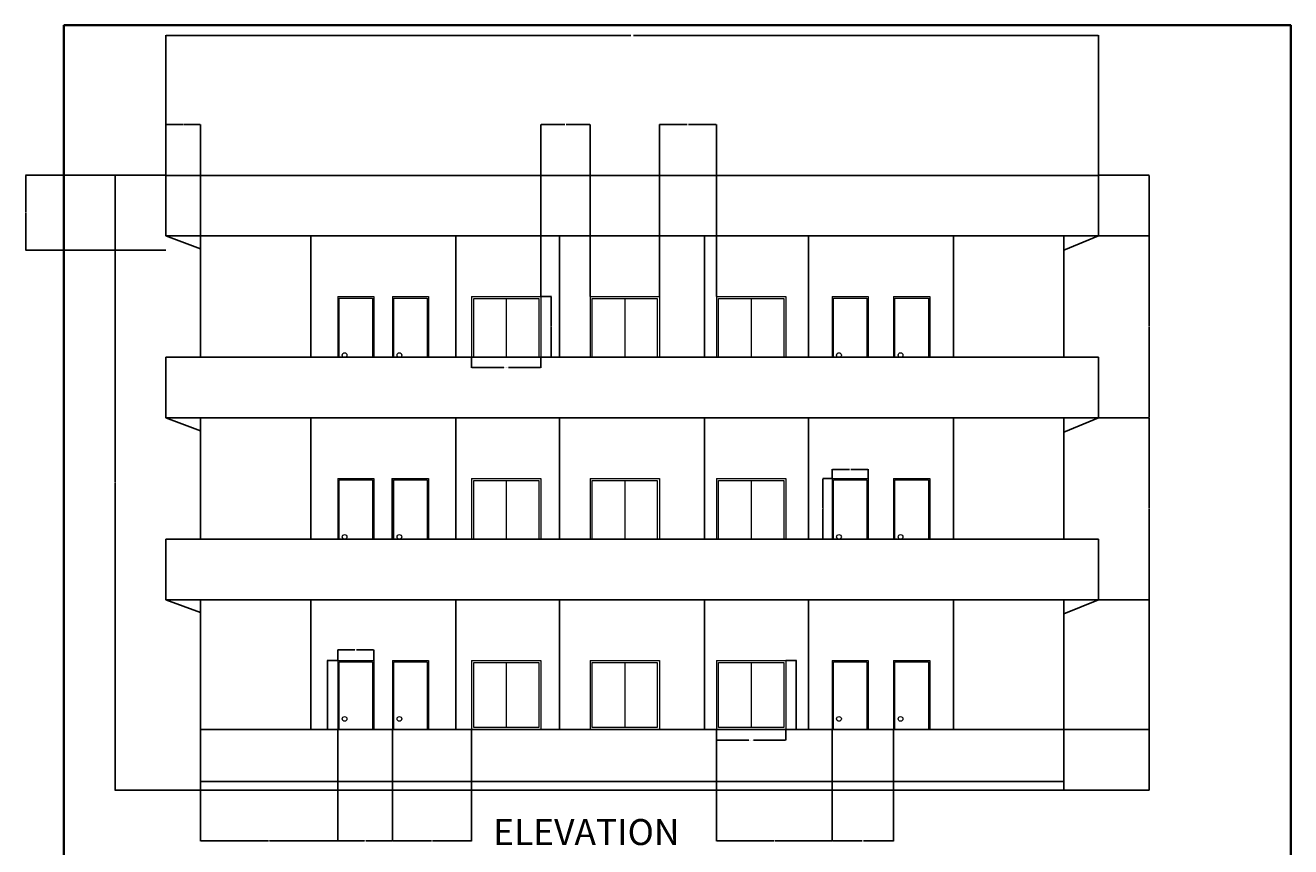
# Model space of a CAD drawing. Units: inches. Extents: x 2165 to 3042, y 1626 to 2968.
# Tile 11 of 11: x 2165 to 3042, y 2399 to 2968. Entities that reach past the tile are written whole.
import ezdxf

# ---------------------------------------------------------------- set-up
doc = ezdxf.new("R2010")
doc.units = ezdxf.units.IN
for name, color, linetype, lineweight in [('A-ANNO-DIMS', 2, 'Continuous', 18), ('A-ANNO-TEXT', 7, 'Continuous', 25), ('A-ELEV', 7, 'Continuous', 25), ('A-ELEV-DOOR', 3, 'Continuous', 18), ('A-ELEV-GLAZ', 4, 'Continuous', 18), ('A-WALL', 7, 'Continuous', 35)]:
    doc.layers.add(name, color=color, linetype=linetype, lineweight=lineweight)
doc.styles.get("Standard").update_dxf_attribs({"font": 'arial.ttf'})
doc.dimstyles.get("Standard").update_dxf_attribs({"dimtxt": 0.18, "dimasz": 0.18, "dimexe": 0.18, "dimexo": 0.0625, "dimgap": 0.09, "dimtad": 0, "dimtih": 1, "dimtoh": 1, "dimdec": 4, "dimzin": 0, "dimdsep": 46, "dimtxsty": 'Standard', "dimcen": 0.09, "dimadec": 0, "dimazin": 0, "dimtfac": 1, "dimtdec": 4, "dimtofl": 0, "dimtmove": 0, "dimatfit": 3, "dimfxl": 1, "dimtolj": 1, "dimtzin": 0, "dimarcsym": 0})

# ---------------------------------------------------------------- blocks, each defined once
blk = doc.blocks.new('ELEV-DOOR-FULL')
for p, q in [((0, 48), (24.97, 48)), ((0, 48), (0, 0)), ((24.97, 48), (24.97, 0))]:
    blk.add_line(p, q)
blk.add_lwpolyline([(0.91, 0), (0.91, 46.97), (24.05, 46.97), (24.05, 0)])
blk.add_circle((4.76, 7.48), 1.64)
blk = doc.blocks.new('ELEV-DOOR-PARTIAL')
for p, q in [((0, 42.16), (24.97, 42.16)), ((0, 42.16), (0, 0.16)), ((24.97, 42.16), (24.97, 0.16))]:
    blk.add_line(p, q)
blk.add_lwpolyline([(0.91, 0.16), (0.91, 41.13), (24.05, 41.13), (24.05, 0.16)])
blk.add_circle((4.76, 1.64), 1.64)
blk = doc.blocks.new('ELEV-WIN-48-SQUARE')
for p, q in [((0, 48), (0, 0)), ((0, 48), (48, 48)), ((24.02, 46.58), (24.02, 1.39)), ((48, 48), (48, 0)), ((0, 0), (48, 0))]:
    blk.add_line(p, q)
blk.add_lwpolyline([(1.46, 46.58), (46.57, 46.58), (46.57, 1.39), (1.46, 1.39)], close=True)
blk = doc.blocks.new('ELEV-WIN-48-PARTIAL')
for p, q in [((0, 42), (0, 0)), ((0, 42), (48, 42)), ((24.02, 40.58), (24.02, 0)), ((48, 42), (48, 0))]:
    blk.add_line(p, q)
blk.add_lwpolyline([(1.46, 0), (1.46, 40.58), (46.57, 40.58), (46.57, 0)])
blk = doc.blocks.new('ELEV-PROJECTING-BAND')
for p, q in [((0, 51.86), (646.5, 51.86)), ((0, 9.86), (0, 51.86)), ((646.5, 9.86), (646.5, 51.86)), ((0, 9.86), (646.5, 9.86)), ((0, 9.86), (24, 0.93)), ((646.5, 9.86), (622.5, 0))]:
    blk.add_line(p, q)
blk = doc.blocks.new('*D40')
at = {"layer": 'A-ANNO-DIMS', "color": 0, "lineweight": -2, "transparency": 16777216}
for p, q in [((2724.42, 2653.94), (2717.98, 2653.94)), ((2718.16, 2653.76), (2718.16, 2633.04)), ((2718.16, 2611.96), (2718.16, 2632.67)), ((2724.42, 2611.78), (2717.98, 2611.78))]:
    blk.add_line(p, q, dxfattribs=at)
at = {"layer": 'A-ANNO-DIMS', "color": 0, "transparency": 16777216}
for points in [[(2718.13, 2653.76), (2718.19, 2653.76), (2718.16, 2653.94)], [(2718.13, 2611.96), (2718.19, 2611.96), (2718.16, 2611.78)]]:
    blk.add_solid(points, dxfattribs=at)
at = {"layer": 'Defpoints', "color": 0, "transparency": 16777216}
for p in [(2718.16, 2653.94), (2724.48, 2653.94), (2724.48, 2611.78)]:
    blk.add_point(p, dxfattribs=at)
at = {"layer": 'A-ANNO-DIMS', "color": 0, "transparency": 16777216, "insert": (2718.16, 2632.86), "char_height": 0.18, "attachment_point": 5}
blk.add_mtext('\\A1;DOOR 42 TYP.', dxfattribs=at)
blk = doc.blocks.new('*D41')
at = {"layer": 'A-ANNO-DIMS', "color": 0, "lineweight": -2, "transparency": 16777216}
for p, q in [((2724.48, 2654), (2724.48, 2660.44)), ((2724.66, 2660.26), (2736.44, 2660.26)), ((2749.27, 2660.26), (2737.5, 2660.26)), ((2749.45, 2654), (2749.45, 2660.44))]:
    blk.add_line(p, q, dxfattribs=at)
at = {"layer": 'A-ANNO-DIMS', "color": 0, "transparency": 16777216}
for points in [[(2724.66, 2660.29), (2724.66, 2660.23), (2724.48, 2660.26)], [(2749.27, 2660.29), (2749.27, 2660.23), (2749.45, 2660.26)]]:
    blk.add_solid(points, dxfattribs=at)
at = {"layer": 'Defpoints', "color": 0, "transparency": 16777216}
for p in [(2749.45, 2660.26), (2724.48, 2653.94), (2749.45, 2653.94)]:
    blk.add_point(p, dxfattribs=at)
at = {"layer": 'A-ANNO-DIMS', "color": 0, "transparency": 16777216, "insert": (2736.97, 2660.26), "char_height": 0.18, "attachment_point": 5}
blk.add_mtext('\\A1;25 TYP.', dxfattribs=at)
blk = doc.blocks.new('*D42')
at = {"layer": 'A-ANNO-DIMS', "color": 0, "lineweight": -2, "transparency": 16777216}
for p, q in [((2474.62, 2737.87), (2474.62, 2730.56)), ((2522.62, 2737.87), (2522.62, 2730.56)), ((2474.8, 2730.74), (2497.04, 2730.74)), ((2522.44, 2730.74), (2500.2, 2730.74))]:
    blk.add_line(p, q, dxfattribs=at)
at = {"layer": 'A-ANNO-DIMS', "color": 0, "transparency": 16777216}
for points in [[(2474.8, 2730.77), (2474.8, 2730.71), (2474.62, 2730.74)], [(2522.44, 2730.77), (2522.44, 2730.71), (2522.62, 2730.74)]]:
    blk.add_solid(points, dxfattribs=at)
at = {"layer": 'Defpoints', "color": 0, "transparency": 16777216}
for p in [(2474.62, 2737.94), (2522.62, 2737.94), (2522.62, 2730.74)]:
    blk.add_point(p, dxfattribs=at)
at = {"layer": 'A-ANNO-DIMS', "color": 0, "transparency": 16777216, "insert": (2498.62, 2730.74), "char_height": 0.18, "attachment_point": 5}
blk.add_mtext('\\A1;UPPER WINDOW 48 TYP.', dxfattribs=at)
blk = doc.blocks.new('*D43')
at = {"layer": 'A-ANNO-DIMS', "color": 0, "lineweight": -2, "transparency": 16777216}
for p, q in [((2522.68, 2779.94), (2530, 2779.94)), ((2529.82, 2779.76), (2529.82, 2759.12)), ((2529.82, 2738.12), (2529.82, 2758.76)), ((2522.68, 2737.94), (2530, 2737.94))]:
    blk.add_line(p, q, dxfattribs=at)
at = {"layer": 'A-ANNO-DIMS', "color": 0, "transparency": 16777216}
for points in [[(2529.79, 2779.76), (2529.85, 2779.76), (2529.82, 2779.94)], [(2529.79, 2738.12), (2529.85, 2738.12), (2529.82, 2737.94)]]:
    blk.add_solid(points, dxfattribs=at)
at = {"layer": 'Defpoints', "color": 0, "transparency": 16777216}
for p in [(2522.62, 2779.94), (2529.82, 2779.94), (2522.62, 2737.94)]:
    blk.add_point(p, dxfattribs=at)
at = {"layer": 'A-ANNO-DIMS', "color": 0, "transparency": 16777216, "insert": (2529.82, 2758.94), "char_height": 0.18, "attachment_point": 5}
blk.add_mtext('\\A1;42 TYP.', dxfattribs=at)
blk = doc.blocks.new('*D44')
at = {"layer": 'A-ANNO-DIMS', "color": 0, "lineweight": -2, "transparency": 16777216}
for p, q in [((2381.72, 2527.94), (2374.41, 2527.94)), ((2374.59, 2527.76), (2374.59, 2504.12)), ((2374.59, 2480.12), (2374.59, 2503.75)), ((2381.72, 2479.94), (2374.41, 2479.94))]:
    blk.add_line(p, q, dxfattribs=at)
at = {"layer": 'A-ANNO-DIMS', "color": 0, "transparency": 16777216}
for points in [[(2374.56, 2527.76), (2374.62, 2527.76), (2374.59, 2527.94)], [(2374.56, 2480.12), (2374.62, 2480.12), (2374.59, 2479.94)]]:
    blk.add_solid(points, dxfattribs=at)
at = {"layer": 'Defpoints', "color": 0, "transparency": 16777216}
for p in [(2374.59, 2527.94), (2381.79, 2527.94), (2381.79, 2479.94)]:
    blk.add_point(p, dxfattribs=at)
at = {"layer": 'A-ANNO-DIMS', "color": 0, "transparency": 16777216, "insert": (2374.59, 2503.94), "char_height": 0.18, "attachment_point": 5}
blk.add_mtext('\\A1;DOOR 48 TYP.', dxfattribs=at)
blk = doc.blocks.new('*D45')
at = {"layer": 'A-ANNO-DIMS', "color": 0, "lineweight": -2, "transparency": 16777216}
for p, q in [((2381.79, 2528), (2381.79, 2535.32)), ((2381.97, 2535.14), (2393.74, 2535.14)), ((2406.57, 2535.14), (2394.8, 2535.14)), ((2406.75, 2528), (2406.75, 2535.32))]:
    blk.add_line(p, q, dxfattribs=at)
at = {"layer": 'A-ANNO-DIMS', "color": 0, "transparency": 16777216}
for points in [[(2381.97, 2535.17), (2381.97, 2535.11), (2381.79, 2535.14)], [(2406.57, 2535.17), (2406.57, 2535.11), (2406.75, 2535.14)]]:
    blk.add_solid(points, dxfattribs=at)
at = {"layer": 'Defpoints', "color": 0, "transparency": 16777216}
for p in [(2406.75, 2535.14), (2381.79, 2527.94), (2406.75, 2527.94)]:
    blk.add_point(p, dxfattribs=at)
at = {"layer": 'A-ANNO-DIMS', "color": 0, "transparency": 16777216, "insert": (2394.27, 2535.14), "char_height": 0.18, "attachment_point": 5}
blk.add_mtext('\\A1;25 TYP.', dxfattribs=at)
blk = doc.blocks.new('*D46')
at = {"layer": 'A-ANNO-DIMS', "color": 0, "lineweight": -2, "transparency": 16777216}
for p, q in [((2644.34, 2479.87), (2644.34, 2472.56)), ((2692.34, 2479.87), (2692.34, 2472.56)), ((2644.52, 2472.74), (2666.73, 2472.74)), ((2692.16, 2472.74), (2669.95, 2472.74))]:
    blk.add_line(p, q, dxfattribs=at)
at = {"layer": 'A-ANNO-DIMS', "color": 0, "transparency": 16777216}
for points in [[(2644.52, 2472.77), (2644.52, 2472.71), (2644.34, 2472.74)], [(2692.16, 2472.77), (2692.16, 2472.71), (2692.34, 2472.74)]]:
    blk.add_solid(points, dxfattribs=at)
at = {"layer": 'Defpoints', "color": 0, "transparency": 16777216}
for p in [(2644.34, 2479.94), (2692.34, 2479.94), (2692.34, 2472.74)]:
    blk.add_point(p, dxfattribs=at)
at = {"layer": 'A-ANNO-DIMS', "color": 0, "transparency": 16777216, "insert": (2668.34, 2472.74), "char_height": 0.18, "attachment_point": 5}
blk.add_mtext('\\A1;LOWER WINDOW 48 TYP.', dxfattribs=at)
blk = doc.blocks.new('*D47')
at = {"layer": 'A-ANNO-DIMS', "color": 0, "lineweight": -2, "transparency": 16777216}
for p, q in [((2692.4, 2527.94), (2699.72, 2527.94)), ((2699.54, 2527.76), (2699.54, 2504.12)), ((2699.54, 2480.12), (2699.54, 2503.75)), ((2692.4, 2479.94), (2699.72, 2479.94))]:
    blk.add_line(p, q, dxfattribs=at)
at = {"layer": 'A-ANNO-DIMS', "color": 0, "transparency": 16777216}
for points in [[(2699.51, 2527.76), (2699.57, 2527.76), (2699.54, 2527.94)], [(2699.51, 2480.12), (2699.57, 2480.12), (2699.54, 2479.94)]]:
    blk.add_solid(points, dxfattribs=at)
at = {"layer": 'Defpoints', "color": 0, "transparency": 16777216}
for p in [(2692.34, 2527.94), (2699.54, 2527.94), (2692.34, 2479.94)]:
    blk.add_point(p, dxfattribs=at)
at = {"layer": 'A-ANNO-DIMS', "color": 0, "transparency": 16777216, "insert": (2699.54, 2503.94), "char_height": 0.18, "attachment_point": 5}
blk.add_mtext('\\A1;48 TYP.', dxfattribs=at)
blk = doc.blocks.new('*D48')
at = {"layer": 'A-ANNO-DIMS', "color": 0, "lineweight": -2, "transparency": 16777216}
for p, q in [((2262.6, 2864), (2262.6, 2961.09)), ((2262.78, 2960.91), (2584.88, 2960.91)), ((2908.92, 2960.91), (2586.83, 2960.91)), ((2909.1, 2864), (2909.1, 2961.09))]:
    blk.add_line(p, q, dxfattribs=at)
at = {"layer": 'A-ANNO-DIMS', "color": 0, "transparency": 16777216}
for points in [[(2262.78, 2960.94), (2262.78, 2960.88), (2262.6, 2960.91)], [(2908.92, 2960.94), (2908.92, 2960.88), (2909.1, 2960.91)]]:
    blk.add_solid(points, dxfattribs=at)
at = {"layer": 'Defpoints', "color": 0, "transparency": 16777216}
for p in [(2909.1, 2960.91), (2262.6, 2863.94), (2909.1, 2863.94)]:
    blk.add_point(p, dxfattribs=at)
at = {"layer": 'A-ANNO-DIMS', "color": 0, "transparency": 16777216, "insert": (2585.85, 2960.91), "char_height": 0.18, "attachment_point": 5}
blk.add_mtext('\\A1;BAND 647 TYP.', dxfattribs=at)
blk = doc.blocks.new('*D49')
at = {"layer": 'A-ANNO-DIMS', "color": 0, "lineweight": -2, "transparency": 16777216}
for p, q in [((2262.54, 2863.94), (2165.45, 2863.94)), ((2165.63, 2863.76), (2165.63, 2838.19)), ((2165.63, 2812.26), (2165.63, 2837.82)), ((2262.54, 2812.08), (2165.45, 2812.08))]:
    blk.add_line(p, q, dxfattribs=at)
at = {"layer": 'A-ANNO-DIMS', "color": 0, "transparency": 16777216}
for points in [[(2165.6, 2863.76), (2165.66, 2863.76), (2165.63, 2863.94)], [(2165.6, 2812.26), (2165.66, 2812.26), (2165.63, 2812.08)]]:
    blk.add_solid(points, dxfattribs=at)
at = {"layer": 'Defpoints', "color": 0, "transparency": 16777216}
for p in [(2165.63, 2863.94), (2262.6, 2863.94), (2262.6, 2812.08)]:
    blk.add_point(p, dxfattribs=at)
at = {"layer": 'A-ANNO-DIMS', "color": 0, "transparency": 16777216, "insert": (2165.63, 2838.01), "char_height": 0.18, "attachment_point": 5}
blk.add_mtext('\\A1;52 TYP.', dxfattribs=at)
blk = doc.blocks.new('*D64')
at = {"layer": 'A-ANNO-DIMS', "color": 0, "lineweight": -2, "transparency": 16777216}
for p, q in [((2262.54, 2863.94), (2227.32, 2863.94)), ((2227.5, 2863.76), (2227.5, 2651.12)), ((2227.5, 2438.12), (2227.5, 2650.75)), ((2286.54, 2437.94), (2227.32, 2437.94))]:
    blk.add_line(p, q, dxfattribs=at)
at = {"layer": 'A-ANNO-DIMS', "color": 0, "transparency": 16777216}
for points in [[(2227.47, 2863.76), (2227.53, 2863.76), (2227.5, 2863.94)], [(2227.47, 2438.12), (2227.53, 2438.12), (2227.5, 2437.94)]]:
    blk.add_solid(points, dxfattribs=at)
at = {"layer": 'Defpoints', "color": 0, "transparency": 16777216}
for p in [(2227.5, 2863.94), (2262.6, 2863.94), (2286.6, 2437.94)]:
    blk.add_point(p, dxfattribs=at)
at = {"layer": 'A-ANNO-DIMS', "color": 0, "transparency": 16777216, "insert": (2227.5, 2650.94), "char_height": 0.18, "attachment_point": 5}
blk.add_mtext('\\A1;426', dxfattribs=at)
blk = doc.blocks.new('*D65')
at = {"layer": 'A-ANNO-DIMS', "color": 0, "lineweight": -2, "transparency": 16777216}
for p, q in [((2885.17, 2479.94), (2944.38, 2479.94)), ((2944.2, 2479.76), (2944.2, 2459.12)), ((2944.2, 2438.12), (2944.2, 2458.76)), ((2885.17, 2437.94), (2944.38, 2437.94))]:
    blk.add_line(p, q, dxfattribs=at)
at = {"layer": 'A-ANNO-DIMS', "color": 0, "transparency": 16777216}
for points in [[(2944.17, 2479.76), (2944.23, 2479.76), (2944.2, 2479.94)], [(2944.17, 2438.12), (2944.23, 2438.12), (2944.2, 2437.94)]]:
    blk.add_solid(points, dxfattribs=at)
at = {"layer": 'Defpoints', "color": 0, "transparency": 16777216}
for p in [(2885.1, 2479.94), (2944.2, 2479.94), (2885.1, 2437.94)]:
    blk.add_point(p, dxfattribs=at)
at = {"layer": 'A-ANNO-DIMS', "color": 0, "transparency": 16777216, "insert": (2944.2, 2458.94), "char_height": 0.18, "attachment_point": 5}
blk.add_mtext('\\A1;42', dxfattribs=at)
blk = doc.blocks.new('*D66')
at = {"layer": 'A-ANNO-DIMS', "color": 0, "lineweight": -2, "transparency": 16777216}
for p, q in [((2909.17, 2569.94), (2944.38, 2569.94)), ((2944.2, 2569.76), (2944.2, 2525.12)), ((2944.2, 2480.12), (2944.2, 2524.75)), ((2885.17, 2479.94), (2944.38, 2479.94))]:
    blk.add_line(p, q, dxfattribs=at)
at = {"layer": 'A-ANNO-DIMS', "color": 0, "transparency": 16777216}
for points in [[(2944.17, 2569.76), (2944.23, 2569.76), (2944.2, 2569.94)], [(2944.17, 2480.12), (2944.23, 2480.12), (2944.2, 2479.94)]]:
    blk.add_solid(points, dxfattribs=at)
at = {"layer": 'Defpoints', "color": 0, "transparency": 16777216}
for p in [(2909.1, 2569.94), (2944.2, 2569.94), (2885.1, 2479.94)]:
    blk.add_point(p, dxfattribs=at)
at = {"layer": 'A-ANNO-DIMS', "color": 0, "transparency": 16777216, "insert": (2944.2, 2524.94), "char_height": 0.18, "attachment_point": 5}
blk.add_mtext('\\A1;90', dxfattribs=at)
blk = doc.blocks.new('*D67')
at = {"layer": 'A-ANNO-DIMS', "color": 0, "lineweight": -2, "transparency": 16777216}
for p, q in [((2909.17, 2695.94), (2944.38, 2695.94)), ((2944.2, 2695.76), (2944.2, 2633.12)), ((2944.2, 2570.12), (2944.2, 2632.75)), ((2909.17, 2569.94), (2944.38, 2569.94))]:
    blk.add_line(p, q, dxfattribs=at)
at = {"layer": 'A-ANNO-DIMS', "color": 0, "transparency": 16777216}
for points in [[(2944.17, 2695.76), (2944.23, 2695.76), (2944.2, 2695.94)], [(2944.17, 2570.12), (2944.23, 2570.12), (2944.2, 2569.94)]]:
    blk.add_solid(points, dxfattribs=at)
at = {"layer": 'Defpoints', "color": 0, "transparency": 16777216}
for p in [(2909.1, 2695.94), (2944.2, 2695.94), (2909.1, 2569.94)]:
    blk.add_point(p, dxfattribs=at)
at = {"layer": 'A-ANNO-DIMS', "color": 0, "transparency": 16777216, "insert": (2944.2, 2632.94), "char_height": 0.18, "attachment_point": 5}
blk.add_mtext('\\A1;126', dxfattribs=at)
blk = doc.blocks.new('*D68')
at = {"layer": 'A-ANNO-DIMS', "color": 0, "lineweight": -2, "transparency": 16777216}
for p, q in [((2909.17, 2821.94), (2944.38, 2821.94)), ((2944.2, 2821.76), (2944.2, 2759.12)), ((2944.2, 2696.12), (2944.2, 2758.75)), ((2909.17, 2695.94), (2944.38, 2695.94))]:
    blk.add_line(p, q, dxfattribs=at)
at = {"layer": 'A-ANNO-DIMS', "color": 0, "transparency": 16777216}
for points in [[(2944.17, 2821.76), (2944.23, 2821.76), (2944.2, 2821.94)], [(2944.17, 2696.12), (2944.23, 2696.12), (2944.2, 2695.94)]]:
    blk.add_solid(points, dxfattribs=at)
at = {"layer": 'Defpoints', "color": 0, "transparency": 16777216}
for p in [(2909.1, 2821.94), (2944.2, 2821.94), (2909.1, 2695.94)]:
    blk.add_point(p, dxfattribs=at)
at = {"layer": 'A-ANNO-DIMS', "color": 0, "transparency": 16777216, "insert": (2944.2, 2758.94), "char_height": 0.18, "attachment_point": 5}
blk.add_mtext('\\A1;126', dxfattribs=at)
blk = doc.blocks.new('*D69')
at = {"layer": 'A-ANNO-DIMS', "color": 0, "lineweight": -2, "transparency": 16777216}
for p, q in [((2909.17, 2863.94), (2944.38, 2863.94)), ((2944.2, 2863.76), (2944.2, 2843.12)), ((2944.2, 2822.12), (2944.2, 2842.76)), ((2909.17, 2821.94), (2944.38, 2821.94))]:
    blk.add_line(p, q, dxfattribs=at)
at = {"layer": 'A-ANNO-DIMS', "color": 0, "transparency": 16777216}
for points in [[(2944.17, 2863.76), (2944.23, 2863.76), (2944.2, 2863.94)], [(2944.17, 2822.12), (2944.23, 2822.12), (2944.2, 2821.94)]]:
    blk.add_solid(points, dxfattribs=at)
at = {"layer": 'Defpoints', "color": 0, "transparency": 16777216}
for p in [(2909.1, 2863.94), (2944.2, 2863.94), (2909.1, 2821.94)]:
    blk.add_point(p, dxfattribs=at)
at = {"layer": 'A-ANNO-DIMS', "color": 0, "transparency": 16777216, "insert": (2944.2, 2842.94), "char_height": 0.18, "attachment_point": 5}
blk.add_mtext('\\A1;42', dxfattribs=at)
blk = doc.blocks.new('*D70')
at = {"layer": 'A-ANNO-DIMS', "color": 0, "lineweight": -2, "transparency": 16777216}
for p, q in [((2262.6, 2822), (2262.6, 2899.22)), ((2262.78, 2899.04), (2274.38, 2899.04)), ((2286.42, 2899.04), (2274.82, 2899.04)), ((2286.6, 2813.07), (2286.6, 2899.22))]:
    blk.add_line(p, q, dxfattribs=at)
at = {"layer": 'A-ANNO-DIMS', "color": 0, "transparency": 16777216}
for points in [[(2262.78, 2899.07), (2262.78, 2899.01), (2262.6, 2899.04)], [(2286.42, 2899.07), (2286.42, 2899.01), (2286.6, 2899.04)]]:
    blk.add_solid(points, dxfattribs=at)
at = {"layer": 'Defpoints', "color": 0, "transparency": 16777216}
for p in [(2286.6, 2899.04), (2262.6, 2821.94), (2286.6, 2813.01)]:
    blk.add_point(p, dxfattribs=at)
at = {"layer": 'A-ANNO-DIMS', "color": 0, "transparency": 16777216, "insert": (2274.6, 2899.04), "char_height": 0.18, "attachment_point": 5}
blk.add_mtext('\\A1;24', dxfattribs=at)
blk = doc.blocks.new('*D71')
at = {"layer": 'A-ANNO-DIMS', "color": 0, "lineweight": -2, "transparency": 16777216}
for p, q in [((2381.79, 2479.87), (2381.79, 2402.66)), ((2286.6, 2437.87), (2286.6, 2402.66)), ((2286.78, 2402.84), (2333.8, 2402.84)), ((2381.61, 2402.84), (2334.59, 2402.84))]:
    blk.add_line(p, q, dxfattribs=at)
at = {"layer": 'A-ANNO-DIMS', "color": 0, "transparency": 16777216}
for points in [[(2286.78, 2402.87), (2286.78, 2402.81), (2286.6, 2402.84)], [(2381.61, 2402.87), (2381.61, 2402.81), (2381.79, 2402.84)]]:
    blk.add_solid(points, dxfattribs=at)
at = {"layer": 'Defpoints', "color": 0, "transparency": 16777216}
for p in [(2381.79, 2479.94), (2286.6, 2437.94), (2381.79, 2402.84)]:
    blk.add_point(p, dxfattribs=at)
at = {"layer": 'A-ANNO-DIMS', "color": 0, "transparency": 16777216, "insert": (2334.19, 2402.84), "char_height": 0.18, "attachment_point": 5}
blk.add_mtext('\\A1;95.18', dxfattribs=at)
blk = doc.blocks.new('*D72')
at = {"layer": 'A-ANNO-DIMS', "color": 0, "lineweight": -2, "transparency": 16777216}
for p, q in [((2381.79, 2479.87), (2381.79, 2402.66)), ((2419.77, 2479.87), (2419.77, 2402.66)), ((2381.97, 2402.84), (2400.38, 2402.84)), ((2419.59, 2402.84), (2401.17, 2402.84))]:
    blk.add_line(p, q, dxfattribs=at)
at = {"layer": 'A-ANNO-DIMS', "color": 0, "transparency": 16777216}
for points in [[(2381.97, 2402.87), (2381.97, 2402.81), (2381.79, 2402.84)], [(2419.59, 2402.87), (2419.59, 2402.81), (2419.77, 2402.84)]]:
    blk.add_solid(points, dxfattribs=at)
at = {"layer": 'Defpoints', "color": 0, "transparency": 16777216}
for p in [(2381.79, 2479.94), (2419.77, 2479.94), (2419.77, 2402.84)]:
    blk.add_point(p, dxfattribs=at)
at = {"layer": 'A-ANNO-DIMS', "color": 0, "transparency": 16777216, "insert": (2400.78, 2402.84), "char_height": 0.18, "attachment_point": 5}
blk.add_mtext('\\A1;37.99', dxfattribs=at)
blk = doc.blocks.new('*D73')
at = {"layer": 'A-ANNO-DIMS', "color": 0, "lineweight": -2, "transparency": 16777216}
for p, q in [((2419.77, 2479.87), (2419.77, 2402.66)), ((2474.62, 2479.87), (2474.62, 2402.66)), ((2419.95, 2402.84), (2446.8, 2402.84)), ((2474.44, 2402.84), (2447.59, 2402.84))]:
    blk.add_line(p, q, dxfattribs=at)
at = {"layer": 'A-ANNO-DIMS', "color": 0, "transparency": 16777216}
for points in [[(2419.95, 2402.87), (2419.95, 2402.81), (2419.77, 2402.84)], [(2474.44, 2402.87), (2474.44, 2402.81), (2474.62, 2402.84)]]:
    blk.add_solid(points, dxfattribs=at)
at = {"layer": 'Defpoints', "color": 0, "transparency": 16777216}
for p in [(2419.77, 2479.94), (2474.62, 2479.94), (2474.62, 2402.84)]:
    blk.add_point(p, dxfattribs=at)
at = {"layer": 'A-ANNO-DIMS', "color": 0, "transparency": 16777216, "insert": (2447.2, 2402.84), "char_height": 0.18, "attachment_point": 5}
blk.add_mtext('\\A1;54.85', dxfattribs=at)
blk = doc.blocks.new('*D74')
at = {"layer": 'A-ANNO-DIMS', "color": 0, "lineweight": -2, "transparency": 16777216}
for p, q in [((2522.62, 2780), (2522.62, 2899.22)), ((2522.8, 2899.04), (2539.21, 2899.04)), ((2556.55, 2899.04), (2540.14, 2899.04)), ((2556.73, 2780), (2556.73, 2899.22))]:
    blk.add_line(p, q, dxfattribs=at)
at = {"layer": 'A-ANNO-DIMS', "color": 0, "transparency": 16777216}
for points in [[(2522.8, 2899.07), (2522.8, 2899.01), (2522.62, 2899.04)], [(2556.55, 2899.07), (2556.55, 2899.01), (2556.73, 2899.04)]]:
    blk.add_solid(points, dxfattribs=at)
at = {"layer": 'Defpoints', "color": 0, "transparency": 16777216}
for p in [(2556.73, 2899.04), (2522.62, 2779.94), (2556.73, 2779.94)]:
    blk.add_point(p, dxfattribs=at)
at = {"layer": 'A-ANNO-DIMS', "color": 0, "transparency": 16777216, "insert": (2539.67, 2899.04), "char_height": 0.18, "attachment_point": 5}
blk.add_mtext('\\A1;34.104', dxfattribs=at)
blk = doc.blocks.new('*D75')
at = {"layer": 'A-ANNO-DIMS', "color": 0, "lineweight": -2, "transparency": 16777216}
for p, q in [((2604.73, 2780), (2604.73, 2899.22)), ((2604.91, 2899.04), (2624.07, 2899.04)), ((2644.16, 2899.04), (2625, 2899.04)), ((2644.34, 2780), (2644.34, 2899.22))]:
    blk.add_line(p, q, dxfattribs=at)
at = {"layer": 'A-ANNO-DIMS', "color": 0, "transparency": 16777216}
for points in [[(2604.91, 2899.07), (2604.91, 2899.01), (2604.73, 2899.04)], [(2644.16, 2899.07), (2644.16, 2899.01), (2644.34, 2899.04)]]:
    blk.add_solid(points, dxfattribs=at)
at = {"layer": 'Defpoints', "color": 0, "transparency": 16777216}
for p in [(2644.34, 2899.04), (2604.73, 2779.94), (2644.34, 2779.94)]:
    blk.add_point(p, dxfattribs=at)
at = {"layer": 'A-ANNO-DIMS', "color": 0, "transparency": 16777216, "insert": (2624.53, 2899.04), "char_height": 0.18, "attachment_point": 5}
blk.add_mtext('\\A1;39.615', dxfattribs=at)
blk = doc.blocks.new('*D76')
at = {"layer": 'A-ANNO-DIMS', "color": 0, "lineweight": -2, "transparency": 16777216}
for p, q in [((2644.34, 2479.87), (2644.34, 2402.66)), ((2724.48, 2479.87), (2724.48, 2402.66)), ((2644.52, 2402.84), (2684.02, 2402.84)), ((2724.3, 2402.84), (2684.81, 2402.84))]:
    blk.add_line(p, q, dxfattribs=at)
at = {"layer": 'A-ANNO-DIMS', "color": 0, "transparency": 16777216}
for points in [[(2644.52, 2402.87), (2644.52, 2402.81), (2644.34, 2402.84)], [(2724.3, 2402.87), (2724.3, 2402.81), (2724.48, 2402.84)]]:
    blk.add_solid(points, dxfattribs=at)
at = {"layer": 'Defpoints', "color": 0, "transparency": 16777216}
for p in [(2644.34, 2479.94), (2724.48, 2479.94), (2724.48, 2402.84)]:
    blk.add_point(p, dxfattribs=at)
at = {"layer": 'A-ANNO-DIMS', "color": 0, "transparency": 16777216, "insert": (2684.41, 2402.84), "char_height": 0.18, "attachment_point": 5}
blk.add_mtext('\\A1;80.14', dxfattribs=at)
blk = doc.blocks.new('*D77')
at = {"layer": 'A-ANNO-DIMS', "color": 0, "lineweight": -2, "transparency": 16777216}
for p, q in [((2724.48, 2479.87), (2724.48, 2402.66)), ((2767.15, 2479.87), (2767.15, 2402.66)), ((2724.66, 2402.84), (2745.42, 2402.84)), ((2766.97, 2402.84), (2746.21, 2402.84))]:
    blk.add_line(p, q, dxfattribs=at)
at = {"layer": 'A-ANNO-DIMS', "color": 0, "transparency": 16777216}
for points in [[(2724.66, 2402.87), (2724.66, 2402.81), (2724.48, 2402.84)], [(2766.97, 2402.87), (2766.97, 2402.81), (2767.15, 2402.84)]]:
    blk.add_solid(points, dxfattribs=at)
at = {"layer": 'Defpoints', "color": 0, "transparency": 16777216}
for p in [(2724.48, 2479.94), (2767.15, 2479.94), (2767.15, 2402.84)]:
    blk.add_point(p, dxfattribs=at)
at = {"layer": 'A-ANNO-DIMS', "color": 0, "transparency": 16777216, "insert": (2745.82, 2402.84), "char_height": 0.18, "attachment_point": 5}
blk.add_mtext('\\A1;42.66', dxfattribs=at)

msp = doc.modelspace()

# ---------------------------------------------------------------- linework, layer by layer
at = {"layer": 'A-ELEV'}
for p, q in [((2286.6045, 2821.9361), (2286.6045, 2737.9361)), ((2363.1045, 2821.9361), (2363.1045, 2737.9361)), ((2463.6045, 2821.9361), (2463.6045, 2737.9361)), ((2535.6045, 2821.9361), (2535.6045, 2737.9361)), ((2636.1045, 2821.9361), (2636.1045, 2737.9361)), ((2708.1045, 2821.9361), (2708.1045, 2737.9361)), ((2708.1045, 2821.9361), (2708.1045, 2737.9361)), ((2808.6045, 2821.9361), (2808.6045, 2737.9361)), ((2808.6045, 2821.9361), (2808.6045, 2737.9361)), ((2885.1045, 2821.9361), (2885.1045, 2737.9361)), ((2286.6045, 2695.9361), (2286.6045, 2611.9361)), ((2286.6045, 2695.9361), (2286.6045, 2689.9361)), ((2363.1045, 2695.9361), (2363.1045, 2611.9361)), ((2463.6045, 2695.9361), (2463.6045, 2611.9361)), ((2535.6045, 2695.9361), (2535.6045, 2611.9361)), ((2636.1045, 2695.9361), (2636.1045, 2611.9361)), ((2708.1045, 2695.9361), (2708.1045, 2611.9361)), ((2708.1045, 2695.9361), (2708.1045, 2611.9361)), ((2808.6045, 2695.9361), (2808.6045, 2611.9361)), ((2808.6045, 2695.9361), (2808.6045, 2611.9361)), ((2885.1045, 2695.9361), (2885.1045, 2611.9361)), ((2885.1045, 2695.9361), (2885.1045, 2689.9361)), ((2286.6045, 2569.9361), (2286.6045, 2437.9361)), ((2286.6045, 2569.9361), (2286.6045, 2563.9361)), ((2363.1045, 2569.9361), (2363.1045, 2479.9361)), ((2463.6045, 2569.9361), (2463.6045, 2479.9361)), ((2535.6045, 2569.9361), (2535.6045, 2479.9361)), ((2636.1045, 2569.9361), (2636.1045, 2479.9361)), ((2708.1045, 2569.9361), (2708.1045, 2479.9361)), ((2708.1045, 2569.9361), (2708.1045, 2479.9361)), ((2808.6045, 2569.9361), (2808.6045, 2479.9361)), ((2808.6045, 2569.9361), (2808.6045, 2479.9361)), ((2885.1045, 2569.9361), (2885.1045, 2437.9361)), ((2885.1045, 2569.9361), (2885.1045, 2563.9361)), ((2363.1045, 2479.9361), (2286.6045, 2479.9361)), ((2286.6045, 2479.9361), (2885.1045, 2479.9361)), ((2363.1045, 2479.9361), (2463.6045, 2479.9361)), ((2708.1045, 2479.9361), (2808.6045, 2479.9361)), ((2286.6045, 2443.9361), (2885.1045, 2443.9361)), ((2286.6045, 2437.9361), (2885.1045, 2437.9361))]:
    msp.add_line(p, q, dxfattribs=at)
at = {"layer": 'A-ELEV-DOOR'}
for p, q in [((2381.7854, 2779.9361), (2406.7549, 2779.9361)), ((2406.7549, 2779.9361), (2406.7549, 2737.9361)), ((2419.7722, 2779.9361), (2444.7417, 2779.9361)), ((2444.7417, 2779.9361), (2444.7417, 2737.9361)), ((2767.1472, 2779.9361), (2792.1167, 2779.9361)), ((2792.1167, 2779.9361), (2792.1167, 2737.9361)), ((2381.7854, 2653.9361), (2406.7549, 2653.9361)), ((2406.7549, 2653.9361), (2406.7549, 2611.9361)), ((2419.2885, 2653.9361), (2419.2885, 2611.9361)), ((2419.2885, 2653.9361), (2444.7417, 2653.9361)), ((2444.7417, 2653.9361), (2444.7417, 2611.9361)), ((2767.1472, 2653.9361), (2792.1167, 2653.9361)), ((2792.1167, 2653.9361), (2792.1167, 2611.9361)), ((2381.7854, 2527.9361), (2406.7549, 2527.9361)), ((2406.7549, 2527.9361), (2406.7549, 2479.9361)), ((2419.7722, 2527.9361), (2444.7417, 2527.9361)), ((2444.7417, 2527.9361), (2444.7417, 2479.9361)), ((2767.1472, 2527.9361), (2792.1167, 2527.9361)), ((2792.1167, 2527.9361), (2792.1167, 2479.9361))]:
    msp.add_line(p, q, dxfattribs=at)
at = {"layer": 'A-ELEV-GLAZ'}
for p, q in [((2556.726, 2779.9361), (2556.726, 2737.9361)), ((2556.726, 2779.9361), (2604.726, 2779.9361)), ((2604.726, 2779.9361), (2604.726, 2737.9361)), ((2644.3411, 2779.9361), (2644.3411, 2737.9361)), ((2644.3411, 2779.9361), (2692.3411, 2779.9361)), ((2692.3411, 2779.9361), (2692.3411, 2737.9361)), ((2556.726, 2653.9361), (2556.726, 2611.9361)), ((2556.726, 2653.9361), (2604.726, 2653.9361)), ((2604.726, 2653.9361), (2604.726, 2611.9361)), ((2644.3411, 2653.9361), (2644.3411, 2611.9361)), ((2644.3411, 2653.9361), (2692.3411, 2653.9361)), ((2692.3411, 2653.9361), (2692.3411, 2611.9361)), ((2556.726, 2527.9361), (2556.726, 2479.9361)), ((2556.726, 2527.9361), (2604.726, 2527.9361)), ((2604.726, 2527.9361), (2604.726, 2479.9361)), ((2644.3411, 2527.9361), (2644.3411, 2479.9361)), ((2644.3411, 2527.9361), (2692.3411, 2527.9361)), ((2692.3411, 2527.9361), (2692.3411, 2479.9361)), ((2556.726, 2479.9361), (2604.726, 2479.9361)), ((2644.3411, 2479.9361), (2692.3411, 2479.9361))]:
    msp.add_line(p, q, dxfattribs=at)
at = {"layer": 'A-WALL'}
msp.add_lwpolyline([(2191.9961, 2967.8547), (3042.3708, 2967.8547), (3042.3708, 1626.3264), (2191.9961, 1626.3264)], close=True, dxfattribs=at)

# ---------------------------------------------------------------- block references
at = {"layer": 'A-ELEV'}
for p in [(2262.604, 2812.076), (2262.604, 2686.076), (2262.604, 2560.076)]:
    msp.add_blockref('ELEV-PROJECTING-BAND', p, dxfattribs=at)
at = {"layer": 'A-ELEV-DOOR'}
for name, p in [('ELEV-DOOR-PARTIAL', (2381.785, 2737.778)), ('ELEV-DOOR-PARTIAL', (2419.7718, 2737.778)), ('ELEV-DOOR-PARTIAL', (2724.4844, 2737.778)), ('ELEV-DOOR-PARTIAL', (2767.1468, 2737.778)), ('ELEV-DOOR-PARTIAL', (2381.785, 2611.778)), ('ELEV-DOOR-PARTIAL', (2419.7718, 2611.778)), ('ELEV-DOOR-PARTIAL', (2724.4844, 2611.778)), ('ELEV-DOOR-PARTIAL', (2767.1468, 2611.778)), ('ELEV-DOOR-FULL', (2381.785, 2479.936)), ('ELEV-DOOR-FULL', (2419.7718, 2479.936)), ('ELEV-DOOR-FULL', (2724.4844, 2479.936)), ('ELEV-DOOR-FULL', (2767.1468, 2479.936))]:
    msp.add_blockref(name, p, dxfattribs=at)
at = {"layer": 'A-ELEV-GLAZ'}
for name, p in [('ELEV-WIN-48-PARTIAL', (2474.622, 2737.936)), ('ELEV-WIN-48-PARTIAL', (2556.726, 2737.936)), ('ELEV-WIN-48-PARTIAL', (2644.3411, 2737.936)), ('ELEV-WIN-48-PARTIAL', (2474.622, 2611.936)), ('ELEV-WIN-48-PARTIAL', (2556.726, 2611.936)), ('ELEV-WIN-48-PARTIAL', (2644.3411, 2611.936)), ('ELEV-WIN-48-SQUARE', (2474.622, 2479.936)), ('ELEV-WIN-48-SQUARE', (2556.726, 2479.936)), ('ELEV-WIN-48-SQUARE', (2644.3411, 2479.936))]:
    msp.add_blockref(name, p, dxfattribs=at)

# ---------------------------------------------------------------- texts
at = {"layer": 'A-ANNO-TEXT', "insert": (2489.5139, 2417.9962), "char_height": 18, "attachment_point": 1}
msp.add_mtext_dynamic_manual_height_columns('ELEVATION', width=440.99545, gutter_width=12.5, heights=[0], dxfattribs=at)

# ---------------------------------------------------------------- dimensions: what is measured, and where the dimension line sits
at = {"layer": 'A-ANNO-DIMS'}
for base, p1, p2, text, picture, middle in [((2909.1044518572, 2960.9110794564), (2262.6044518572, 2863.9360794564), (2909.1044518572, 2863.9360794564), 'BAND <> TYP.', '*D48', (2585.8544518572, 2960.9110794564)), ((2522.622, 2730.7361), (2474.622, 2737.9361), (2522.622, 2737.9361), 'UPPER WINDOW <> TYP.', '*D42', (2498.622, 2730.7361)), ((2749.4543, 2660.2597), (2724.4848, 2653.9361), (2749.4543, 2653.9361), '<> TYP.', '*D41', (2736.9695, 2660.2597)), ((2406.7549, 2535.1361), (2381.7854, 2527.9361), (2406.7549, 2527.9361), '<> TYP.', '*D45', (2394.2701, 2535.1361)), ((2692.3411, 2472.7361), (2644.3411, 2479.9361), (2692.3411, 2479.9361), 'LOWER WINDOW <> TYP.', '*D46', (2668.3411, 2472.7361))]:
    dim = msp.add_linear_dim(base=base, p1=p1, p2=p2, text=text, dimstyle='Standard', override={"dimdec": 0, "dimlfac": 1, "dimrnd": 0, "dimzin": 0, "dimdsep": 46, "dimlunit": 2}, dxfattribs=at)
    dim.commit()
    dim.dimension.update_dxf_attribs({"geometry": picture, "text_midpoint": middle})
for base, p1, p2, override, picture, middle in [((2286.6045, 2899.0361), (2262.6045, 2821.9361), (2286.6045, 2813.0064), {"dimdec": 0, "dimlfac": 1, "dimrnd": 0, "dimzin": 0, "dimdsep": 46, "dimlunit": 2}, '*D70', (2274.6045, 2899.0361)), ((2556.726, 2899.0361), (2522.622, 2779.9361), (2556.726, 2779.9361), {"dimdec": 3, "dimlfac": 1, "dimrnd": 0, "dimzin": 0, "dimdsep": 46, "dimlunit": 2}, '*D74', (2539.674, 2899.0361)), ((2644.3411, 2899.0361), (2604.726, 2779.9361), (2644.3411, 2779.9361), {"dimdec": 3, "dimlfac": 1, "dimrnd": 0, "dimzin": 0, "dimdsep": 46, "dimlunit": 2}, '*D75', (2624.5336, 2899.0361)), ((2381.7854, 2402.8361), (2286.6045, 2437.9361), (2381.7854, 2479.9361), {"dimdec": 2, "dimlfac": 1, "dimrnd": 0, "dimzin": 0, "dimdsep": 46, "dimlunit": 2}, '*D71', (2334.1949, 2402.8361)), ((2419.7722, 2402.8361), (2381.7854, 2479.9361), (2419.7722, 2479.9361), {"dimdec": 2, "dimlfac": 1, "dimrnd": 0, "dimzin": 0, "dimdsep": 46, "dimlunit": 2}, '*D72', (2400.7788, 2402.8361)), ((2474.622, 2402.8361), (2419.7722, 2479.9361), (2474.622, 2479.9361), {"dimdec": 2, "dimlfac": 1, "dimrnd": 0, "dimzin": 0, "dimdsep": 46, "dimlunit": 2}, '*D73', (2447.1971, 2402.8361)), ((2724.4848, 2402.8361), (2644.3411, 2479.9361), (2724.4848, 2479.9361), {"dimdec": 2, "dimlfac": 1, "dimrnd": 0, "dimzin": 0, "dimdsep": 46, "dimlunit": 2}, '*D76', (2684.413, 2402.8361)), ((2767.1472, 2402.8361), (2724.4848, 2479.9361), (2767.1472, 2479.9361), {"dimdec": 2, "dimlfac": 1, "dimrnd": 0, "dimzin": 0, "dimdsep": 46, "dimlunit": 2}, '*D77', (2745.816, 2402.8361))]:
    dim = msp.add_linear_dim(base=base, p1=p1, p2=p2, dimstyle='Standard', override=override, dxfattribs=at)
    dim.commit()
    dim.dimension.update_dxf_attribs({"geometry": picture, "text_midpoint": middle})
for base, p1, p2, text, picture, middle in [((2165.6295, 2863.9361), (2262.6045, 2812.0755), (2262.6045, 2863.9361), '<> TYP.', '*D49', (2165.6295, 2838.0058)), ((2529.822, 2779.9361), (2522.622, 2737.9361), (2522.622, 2779.9361), '<> TYP.', '*D43', (2529.822, 2758.9361)), ((2718.1611, 2653.9361), (2724.4848, 2611.7784), (2724.4848, 2653.9361), 'DOOR <> TYP.', '*D40', (2718.1611, 2632.8573)), ((2374.5854, 2527.9361), (2381.7854, 2479.9361), (2381.7854, 2527.9361), 'DOOR <> TYP.', '*D44', (2374.5854, 2503.9361)), ((2699.5411, 2527.9361), (2692.3411, 2479.9361), (2692.3411, 2527.9361), '<> TYP.', '*D47', (2699.5411, 2503.9361))]:
    dim = msp.add_linear_dim(base=base, p1=p1, p2=p2, angle=90, text=text, dimstyle='Standard', override={"dimdec": 0, "dimlfac": 1, "dimrnd": 0, "dimzin": 0, "dimdsep": 46, "dimlunit": 2}, dxfattribs=at)
    dim.commit()
    dim.dimension.update_dxf_attribs({"geometry": picture, "text_midpoint": middle})
for base, p1, p2, picture, middle in [((2227.5045, 2863.9361), (2286.6045, 2437.9361), (2262.6045, 2863.9361), '*D64', (2227.5045, 2650.9361)), ((2944.2045, 2863.9361), (2909.1045, 2821.9361), (2909.1045, 2863.9361), '*D69', (2944.2045, 2842.9361)), ((2944.2045, 2821.9361), (2909.1045, 2695.9361), (2909.1045, 2821.9361), '*D68', (2944.2045, 2758.9361)), ((2944.2045, 2695.9361), (2909.1045, 2569.9361), (2909.1045, 2695.9361), '*D67', (2944.2045, 2632.9361)), ((2944.2045, 2569.9361), (2885.1045, 2479.9361), (2909.1045, 2569.9361), '*D66', (2944.2045, 2524.9361)), ((2944.2045, 2479.9361), (2885.1045, 2437.9361), (2885.1045, 2479.9361), '*D65', (2944.2045, 2458.9361))]:
    dim = msp.add_linear_dim(base=base, p1=p1, p2=p2, angle=90, dimstyle='Standard', override={"dimdec": 0, "dimlfac": 1, "dimrnd": 0, "dimzin": 0, "dimdsep": 46, "dimlunit": 2}, dxfattribs=at)
    dim.commit()
    dim.dimension.update_dxf_attribs({"geometry": picture, "text_midpoint": middle})

doc.saveas('drawing.dxf')
